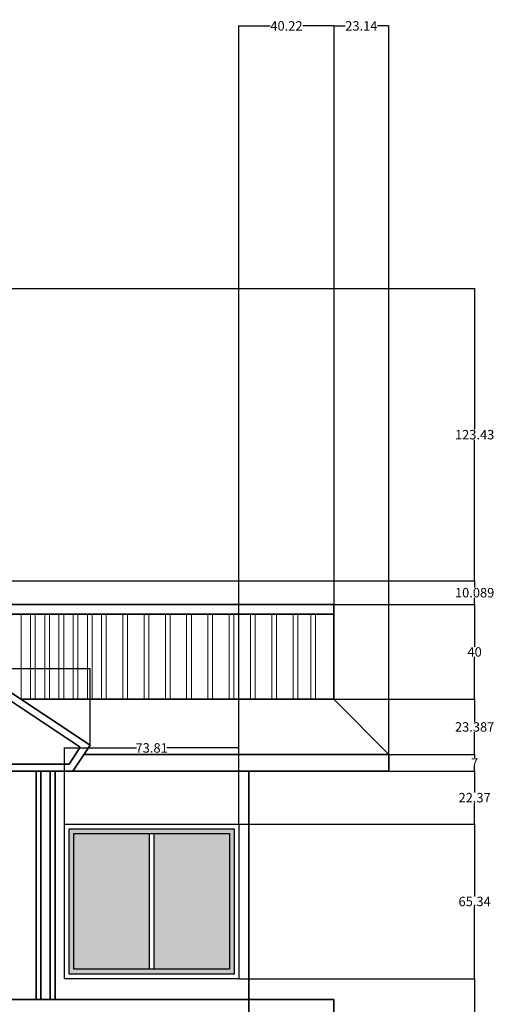
# Model space of a CAD drawing. Units: inches. Extents: x 1366 to 1929, y 372 to 1068.
# Tile 4 of 4: x 1728 to 1929, y 652 to 1068. Entities that reach past the tile are written whole.
import ezdxf

# ---------------------------------------------------------------- set-up
doc = ezdxf.new("R2010")
doc.units = ezdxf.units.IN
doc.header["$MEASUREMENT"] = 0
for name, color, linetype, lineweight in [('A-ANNO-DIMS', 2, 'Continuous', 18), ('A-ELEV', 7, 'Continuous', 35), ('A-ELEV-PATT', 252, 'Continuous', 13), ('A-ELEV-RAIL', 8, 'Continuous', 18), ('A-GLAZ', 4, 'Continuous', 30)]:
    doc.layers.add(name, color=color, linetype=linetype, lineweight=lineweight)
doc.styles.get("Standard").update_dxf_attribs({"font": 'arial.ttf'})
doc.dimstyles.get("Standard").update_dxf_attribs({"dimtxt": 4, "dimasz": 0.18, "dimexe": 0.18, "dimexo": 0.0625, "dimgap": 0.09, "dimtad": 0, "dimtih": 1, "dimtoh": 1, "dimdec": 0, "dimrnd": 6, "dimzin": 0, "dimdsep": 46, "dimlunit": 3, "dimtxsty": 'Standard', "dimcen": 0.09, "dimadec": 0, "dimazin": 0, "dimtfac": 1, "dimtdec": 0, "dimtofl": 0, "dimtmove": 0, "dimatfit": 3, "dimfxl": 1, "dimtolj": 1, "dimtzin": 0, "dimarcsym": 0})

# ---------------------------------------------------------------- blocks, each defined once
blk = doc.blocks.new('*D16')
at = {"layer": 'A-ANNO-DIMS', "color": 0, "lineweight": -2, "transparency": 16777216}
for p, q in [((1820.72, 727.69), (1820.72, 1065.06)), ((1860.94, 820.44), (1860.94, 1065.06)), ((1820.9, 1064.88), (1833.93, 1064.88)), ((1860.76, 1064.88), (1847.73, 1064.88))]:
    blk.add_line(p, q, dxfattribs=at)
at = {"layer": 'A-ANNO-DIMS', "color": 0, "lineweight": 30, "transparency": 16777216}
for points in [[(1820.9, 1064.91), (1820.9, 1064.85), (1820.72, 1064.88)], [(1860.76, 1064.91), (1860.76, 1064.85), (1860.94, 1064.88)]]:
    blk.add_solid(points, dxfattribs=at)
at = {"layer": 'Defpoints', "color": 0, "lineweight": 30, "transparency": 16777216}
for p in [(1860.94, 1064.88), (1860.94, 820.38), (1820.72, 727.62)]:
    blk.add_point(p, dxfattribs=at)
at = {"layer": 'A-ANNO-DIMS', "color": 0, "transparency": 16777216, "insert": (1840.83, 1064.88), "char_height": 4, "attachment_point": 5}
blk.add_mtext('\\A1;40.22', dxfattribs=at)
blk = doc.blocks.new('*D17')
at = {"layer": 'A-ANNO-DIMS', "color": 0, "lineweight": -2, "transparency": 16777216}
for p, q in [((1860.94, 820.44), (1860.94, 1065.06)), ((1884.08, 757.06), (1884.08, 1065.06)), ((1861.12, 1064.88), (1865.64, 1064.88)), ((1883.9, 1064.88), (1879.37, 1064.88))]:
    blk.add_line(p, q, dxfattribs=at)
at = {"layer": 'A-ANNO-DIMS', "color": 0, "lineweight": 30, "transparency": 16777216}
for points in [[(1861.12, 1064.91), (1861.12, 1064.85), (1860.94, 1064.88)], [(1883.9, 1064.91), (1883.9, 1064.85), (1884.08, 1064.88)]]:
    blk.add_solid(points, dxfattribs=at)
at = {"layer": 'Defpoints', "color": 0, "lineweight": 30, "transparency": 16777216}
for p in [(1884.08, 1064.88), (1860.94, 820.38), (1884.08, 756.99)]:
    blk.add_point(p, dxfattribs=at)
at = {"layer": 'A-ANNO-DIMS', "color": 0, "transparency": 16777216, "insert": (1872.51, 1064.88), "char_height": 4, "attachment_point": 5}
blk.add_mtext('\\A1;23.14', dxfattribs=at)
blk = doc.blocks.new('*D43')
at = {"layer": 'A-ANNO-DIMS', "color": 0, "lineweight": -2, "transparency": 16777216}
for p, q in [((1820.78, 662.28), (1920.61, 662.28)), ((1920.43, 662.1), (1920.43, 626.24)), ((1920.43, 586.11), (1920.43, 621.97)), ((1888.28, 585.93), (1920.61, 585.93))]:
    blk.add_line(p, q, dxfattribs=at)
at = {"layer": 'A-ANNO-DIMS', "color": 0, "lineweight": 30, "transparency": 16777216}
for points in [[(1920.4, 662.1), (1920.46, 662.1), (1920.43, 662.28)], [(1920.4, 586.11), (1920.46, 586.11), (1920.43, 585.93)]]:
    blk.add_solid(points, dxfattribs=at)
at = {"layer": 'Defpoints', "color": 0, "lineweight": 30, "transparency": 16777216}
for p in [(1820.72, 662.28), (1920.43, 662.28), (1888.22, 585.93)]:
    blk.add_point(p, dxfattribs=at)
at = {"layer": 'A-ANNO-DIMS', "color": 0, "transparency": 16777216, "insert": (1920.43, 624.11), "char_height": 4, "attachment_point": 5}
blk.add_mtext('\\A1;76.35', dxfattribs=at)
blk = doc.blocks.new('*D44')
at = {"layer": 'A-ANNO-DIMS', "color": 0, "lineweight": -2, "transparency": 16777216}
for p, q in [((1820.78, 727.62), (1920.61, 727.62)), ((1920.43, 727.44), (1920.43, 697.09)), ((1920.43, 662.46), (1920.43, 692.82)), ((1820.78, 662.28), (1920.61, 662.28))]:
    blk.add_line(p, q, dxfattribs=at)
at = {"layer": 'A-ANNO-DIMS', "color": 0, "lineweight": 30, "transparency": 16777216}
for points in [[(1920.4, 727.44), (1920.46, 727.44), (1920.43, 727.62)], [(1920.4, 662.46), (1920.46, 662.46), (1920.43, 662.28)]]:
    blk.add_solid(points, dxfattribs=at)
at = {"layer": 'Defpoints', "color": 0, "lineweight": 30, "transparency": 16777216}
for p in [(1820.72, 727.62), (1920.43, 727.62), (1820.72, 662.28)]:
    blk.add_point(p, dxfattribs=at)
at = {"layer": 'A-ANNO-DIMS', "color": 0, "transparency": 16777216, "insert": (1920.43, 694.95), "char_height": 4, "attachment_point": 5}
blk.add_mtext('\\A1;65.34', dxfattribs=at)
blk = doc.blocks.new('*D45')
at = {"layer": 'A-ANNO-DIMS', "color": 0, "lineweight": -2, "transparency": 16777216}
for p, q in [((1884.14, 749.99), (1920.61, 749.99)), ((1920.43, 749.81), (1920.43, 740.94)), ((1920.43, 727.8), (1920.43, 736.67)), ((1820.78, 727.62), (1920.61, 727.62))]:
    blk.add_line(p, q, dxfattribs=at)
at = {"layer": 'A-ANNO-DIMS', "color": 0, "lineweight": 30, "transparency": 16777216}
for points in [[(1920.4, 749.81), (1920.46, 749.81), (1920.43, 749.99)], [(1920.4, 727.8), (1920.46, 727.8), (1920.43, 727.62)]]:
    blk.add_solid(points, dxfattribs=at)
at = {"layer": 'Defpoints', "color": 0, "lineweight": 30, "transparency": 16777216}
for p in [(1884.08, 749.99), (1920.43, 749.99), (1820.72, 727.62)]:
    blk.add_point(p, dxfattribs=at)
at = {"layer": 'A-ANNO-DIMS', "color": 0, "transparency": 16777216, "insert": (1920.43, 738.81), "char_height": 4, "attachment_point": 5}
blk.add_mtext('\\A1;22.37', dxfattribs=at)
blk = doc.blocks.new('*D46')
at = {"layer": 'A-ANNO-DIMS', "color": 0, "lineweight": -2, "transparency": 16777216}
for p, q in [((1884.139646, 756.992679), (1920.609691, 756.992679)), ((1920.429691, 756.812679), (1920.429691, 755.582679)), ((1884.139646, 749.992679), (1920.609691, 749.992679)), ((1920.429691, 750.172679), (1920.429691, 751.402679))]:
    blk.add_line(p, q, dxfattribs=at)
at = {"layer": 'A-ANNO-DIMS', "color": 0, "lineweight": 30, "transparency": 16777216}
for points in [[(1920.399691, 756.812679), (1920.459691, 756.812679), (1920.429691, 756.992679)], [(1920.399691, 750.172679), (1920.459691, 750.172679), (1920.429691, 749.992679)]]:
    blk.add_solid(points, dxfattribs=at)
at = {"layer": 'Defpoints', "color": 0, "lineweight": 30, "transparency": 16777216}
for p in [(1884.077146, 756.992679), (1920.429691, 756.992679), (1884.077146, 749.992679)]:
    blk.add_point(p, dxfattribs=at)
at = {"layer": 'A-ANNO-DIMS', "color": 0, "transparency": 16777216, "insert": (1920.429691, 753.492679), "char_height": 4, "attachment_point": 5}
blk.add_mtext('\\A1;7', dxfattribs=at)
blk = doc.blocks.new('*D47')
at = {"layer": 'A-ANNO-DIMS', "color": 0, "lineweight": -2, "transparency": 16777216}
for p, q in [((1861, 780.38), (1920.61, 780.38)), ((1920.43, 780.2), (1920.43, 770.82)), ((1920.43, 757.17), (1920.43, 766.55)), ((1884.14, 756.99), (1920.61, 756.99))]:
    blk.add_line(p, q, dxfattribs=at)
at = {"layer": 'A-ANNO-DIMS', "color": 0, "lineweight": 30, "transparency": 16777216}
for points in [[(1920.4, 780.2), (1920.46, 780.2), (1920.43, 780.38)], [(1920.4, 757.17), (1920.46, 757.17), (1920.43, 756.99)]]:
    blk.add_solid(points, dxfattribs=at)
at = {"layer": 'Defpoints', "color": 0, "lineweight": 30, "transparency": 16777216}
for p in [(1860.94, 780.38), (1920.43, 780.38), (1884.08, 756.99)]:
    blk.add_point(p, dxfattribs=at)
at = {"layer": 'A-ANNO-DIMS', "color": 0, "transparency": 16777216, "insert": (1920.43, 768.69), "char_height": 4, "attachment_point": 5}
blk.add_mtext('\\A1;23.387', dxfattribs=at)
blk = doc.blocks.new('*D48')
at = {"layer": 'A-ANNO-DIMS', "color": 0, "lineweight": -2, "transparency": 16777216}
for p, q in [((1861, 820.38), (1920.61, 820.38)), ((1920.43, 820.2), (1920.43, 802.51)), ((1920.43, 780.56), (1920.43, 798.25)), ((1861, 780.38), (1920.61, 780.38))]:
    blk.add_line(p, q, dxfattribs=at)
at = {"layer": 'A-ANNO-DIMS', "color": 0, "lineweight": 30, "transparency": 16777216}
for points in [[(1920.4, 820.2), (1920.46, 820.2), (1920.43, 820.38)], [(1920.4, 780.56), (1920.46, 780.56), (1920.43, 780.38)]]:
    blk.add_solid(points, dxfattribs=at)
at = {"layer": 'Defpoints', "color": 0, "lineweight": 30, "transparency": 16777216}
for p in [(1860.94, 820.38), (1920.43, 820.38), (1860.94, 780.38)]:
    blk.add_point(p, dxfattribs=at)
at = {"layer": 'A-ANNO-DIMS', "color": 0, "transparency": 16777216, "insert": (1920.43, 800.38), "char_height": 4, "attachment_point": 5}
blk.add_mtext('\\A1;40', dxfattribs=at)
blk = doc.blocks.new('*D49')
at = {"layer": 'A-ANNO-DIMS', "color": 0, "lineweight": -2, "transparency": 16777216}
for p, q in [((1652.94, 830.47), (1920.61, 830.47)), ((1920.43, 830.29), (1920.43, 827.56)), ((1861, 820.38), (1920.61, 820.38)), ((1920.43, 820.56), (1920.43, 823.29))]:
    blk.add_line(p, q, dxfattribs=at)
at = {"layer": 'A-ANNO-DIMS', "color": 0, "lineweight": 30, "transparency": 16777216}
for points in [[(1920.4, 830.29), (1920.46, 830.29), (1920.43, 830.47)], [(1920.4, 820.56), (1920.46, 820.56), (1920.43, 820.38)]]:
    blk.add_solid(points, dxfattribs=at)
at = {"layer": 'Defpoints', "color": 0, "lineweight": 30, "transparency": 16777216}
for p in [(1652.88, 830.47), (1920.43, 830.47), (1860.94, 820.38)]:
    blk.add_point(p, dxfattribs=at)
at = {"layer": 'A-ANNO-DIMS', "color": 0, "transparency": 16777216, "insert": (1920.43, 825.42), "char_height": 4, "attachment_point": 5}
blk.add_mtext('\\A1;10.089', dxfattribs=at)
blk = doc.blocks.new('*D50')
at = {"layer": 'A-ANNO-DIMS', "color": 0, "lineweight": -2, "transparency": 16777216}
for p, q in [((1651.18, 953.9), (1920.61, 953.9)), ((1920.43, 953.72), (1920.43, 894.32)), ((1920.43, 830.65), (1920.43, 890.05)), ((1652.94, 830.47), (1920.61, 830.47))]:
    blk.add_line(p, q, dxfattribs=at)
at = {"layer": 'A-ANNO-DIMS', "color": 0, "lineweight": 30, "transparency": 16777216}
for points in [[(1920.4, 953.72), (1920.46, 953.72), (1920.43, 953.9)], [(1920.4, 830.65), (1920.46, 830.65), (1920.43, 830.47)]]:
    blk.add_solid(points, dxfattribs=at)
at = {"layer": 'Defpoints', "color": 0, "lineweight": 30, "transparency": 16777216}
for p in [(1651.11, 953.9), (1920.43, 953.9), (1652.88, 830.47)]:
    blk.add_point(p, dxfattribs=at)
at = {"layer": 'A-ANNO-DIMS', "color": 0, "transparency": 16777216, "insert": (1920.43, 892.18), "char_height": 4, "attachment_point": 5}
blk.add_mtext('\\A1;123.43', dxfattribs=at)
blk = doc.blocks.new('*D51')
at = {"layer": 'A-ANNO-DIMS', "color": 0, "lineweight": -2, "transparency": 16777216}
for p, q in [((1746.91, 727.69), (1746.91, 760)), ((1747.09, 759.82), (1777.38, 759.82)), ((1820.54, 759.82), (1790.25, 759.82)), ((1820.72, 727.69), (1820.72, 760))]:
    blk.add_line(p, q, dxfattribs=at)
at = {"layer": 'A-ANNO-DIMS', "color": 0, "lineweight": 30, "transparency": 16777216}
for points in [[(1747.09, 759.85), (1747.09, 759.79), (1746.91, 759.82)], [(1820.54, 759.85), (1820.54, 759.79), (1820.72, 759.82)]]:
    blk.add_solid(points, dxfattribs=at)
at = {"layer": 'Defpoints', "color": 0, "lineweight": 30, "transparency": 16777216}
for p in [(1820.72, 759.82), (1746.91, 727.62), (1820.72, 727.62)]:
    blk.add_point(p, dxfattribs=at)
at = {"layer": 'A-ANNO-DIMS', "color": 0, "transparency": 16777216, "insert": (1783.81, 759.82), "char_height": 4, "attachment_point": 5}
blk.add_mtext('\\A1;73.81', dxfattribs=at)
blk = doc.blocks.new('*D62')
at = {"layer": 'A-ANNO-DIMS', "color": 0, "lineweight": -2, "transparency": 16777216}
for p, q in [((1547.72, 761.06), (1547.72, 793.37)), ((1547.9, 793.19), (1644.33, 793.19)), ((1757.61, 793.19), (1661.18, 793.19)), ((1757.79, 761.06), (1757.79, 793.37))]:
    blk.add_line(p, q, dxfattribs=at)
at = {"layer": 'A-ANNO-DIMS', "color": 0, "lineweight": 30, "transparency": 16777216}
for points in [[(1547.9, 793.22), (1547.9, 793.16), (1547.72, 793.19)], [(1757.61, 793.22), (1757.61, 793.16), (1757.79, 793.19)]]:
    blk.add_solid(points, dxfattribs=at)
at = {"layer": 'Defpoints', "color": 0, "lineweight": 30, "transparency": 16777216}
for p in [(1757.79, 793.19), (1547.72, 760.99), (1757.79, 760.99)]:
    blk.add_point(p, dxfattribs=at)
at = {"layer": 'A-ANNO-DIMS', "color": 0, "transparency": 16777216, "insert": (1652.75, 793.19), "char_height": 4, "attachment_point": 5}
blk.add_mtext('\\A1;210.06', dxfattribs=at)

msp = doc.modelspace()

# ---------------------------------------------------------------- hatches: boundary and pattern name
at = {"layer": 'A-ELEV-PATT'}
h = msp.add_hatch(color=256, dxfattribs=at)
h.dxf.hatch_style = 1
h.paths.add_polyline_path([(1546.6356, 729.6227), (1468.827, 729.6227), (1468.827, 660.2826), (1546.6356, 660.2826)])
h.paths.add_polyline_path([(1544.6356, 662.2826), (1470.827, 662.2826), (1470.827, 727.6227), (1544.6356, 727.6227)], flags=16)
h.paths.add_polyline_path([(1818.7172, 725.6227), (1748.9085, 725.6227), (1748.9085, 664.2826), (1818.7172, 664.2826)])
h.paths.add_polyline_path([(1750.9085, 723.6227), (1816.7172, 723.6227), (1816.7172, 666.2826), (1750.9085, 666.2826)], flags=16)
h.paths.add_polyline_path([(1546.6356, 895.5665), (1468.827, 895.5665), (1468.827, 826.2264), (1546.6356, 826.2264)])
h.paths.add_polyline_path([(1544.6356, 828.2264), (1470.827, 828.2264), (1470.827, 893.5665), (1544.6356, 893.5665)], flags=16)
h = msp.add_hatch(dxfattribs=at)
h.set_pattern_fill('ANGLE', color=256, scale=25)
h.set_pattern_definition([(0, (0, 0), (0, 6.875), [5, -1.875]), (90, (0, 0), (-6.875, 4e-16), [5, -1.875])])
h.paths.add_polyline_path([(1544.6356, 893.5665), (1508.6356, 893.5665), (1508.6356, 828.2264), (1544.6356, 828.2264)])
h.paths.add_polyline_path([(1506.6356, 727.6227), (1470.827, 727.6227), (1470.827, 662.2826), (1506.6356, 662.2826)])
h.paths.add_polyline_path([(1544.6356, 727.6227), (1508.6356, 727.6227), (1508.6356, 662.2826), (1544.6356, 662.2826)])
h.paths.add_polyline_path([(1608.5338, 752.9927), (1697.2248, 752.9927, 0.93463511)])
h.paths.add_polyline_path([(1682.8585, 567.593), (1622.7881, 567.593), (1622.7881, 535.593), (1682.8585, 535.593)])
h.paths.add_polyline_path([(1782.7172, 723.6227), (1750.9085, 723.6227), (1750.9085, 666.2826), (1782.7172, 666.2826)])
h.paths.add_polyline_path([(1816.7172, 723.6227), (1784.7172, 723.6227), (1784.7172, 666.2826), (1816.7172, 666.2826)])
h.paths.add_polyline_path([(1817.1901, 526.1862), (1739.2847, 526.1862), (1739.2847, 513.1136), (1817.1901, 513.1136)])
h.paths.add_polyline_path([(1565.633, 526.1862), (1487.7276, 526.1862), (1487.7276, 513.1136), (1565.633, 513.1136)])

# ---------------------------------------------------------------- linework, layer by layer
at = {"layer": 'A-ELEV'}
for p, q in [((1652.8793, 830.4686), (1757.7853, 760.9927)), ((1652.8773, 826.8716), (1753.6243, 760.1501)), ((1668.1133, 820.3796), (1860.9351, 820.3796)), ((1860.9351, 820.3796), (1860.9351, 780.3796)), ((1860.9351, 820.3796), (1860.9351, 780.3796)), ((1674.1531, 816.3796), (1860.9351, 816.3796)), ((1728.5118, 780.3796), (1860.9351, 780.3796)), ((1860.9351, 780.3796), (1884.0771, 756.9927)), ((1755.2863, 762.6525), (1755.284, 762.6492)), ((1753.6243, 760.1501), (1748.8704, 752.9927)), ((1757.7853, 760.9927), (1750.4793, 749.9927)), ((1756.1255, 758.4937), (1756.1288, 758.4915)), ((1703.2369, 752.9927), (1748.8704, 752.9927)), ((1755.1285, 756.9927), (1884.0771, 756.9927)), ((1884.0771, 756.9927), (1884.0771, 749.9927)), ((1439.2218, 749.9927), (1860.9351, 749.9927)), ((1734.9351, 749.9927), (1734.9351, 653.5057)), ((1736.9351, 749.9927), (1736.9351, 653.5057)), ((1740.9351, 749.9927), (1740.9351, 653.5057)), ((1742.9351, 749.9927), (1742.9351, 653.5057)), ((1824.9351, 749.9927), (1824.9351, 613.5057)), ((1860.9351, 749.9927), (1884.0771, 749.9927)), ((1439.2218, 653.5057), (1860.9351, 653.5057)), ((1860.9351, 653.5057), (1860.9351, 613.5057))]:
    msp.add_line(p, q, dxfattribs=at)
at = {"layer": 'A-ELEV-RAIL'}
for p, q in [((1728.6001, 816.3796), (1728.6001, 780.3796)), ((1732.6001, 816.3796), (1732.6001, 780.3796)), ((1734.6001, 816.3796), (1734.6001, 780.3796)), ((1738.6001, 816.3796), (1738.6001, 780.3796)), ((1740.6001, 816.3796), (1740.6001, 780.3796)), ((1744.6001, 816.3796), (1744.6001, 780.3796)), ((1746.6001, 816.3796), (1746.6001, 780.3796)), ((1750.6001, 816.3796), (1750.6001, 780.3796)), ((1752.6001, 816.3796), (1752.6001, 780.3796)), ((1756.6001, 816.3796), (1756.6001, 780.3796)), ((1758.6001, 816.3796), (1758.6001, 780.3796)), ((1762.6001, 816.3796), (1762.6001, 780.3796)), ((1764.6001, 816.3796), (1764.6001, 780.3796)), ((1771.6001, 816.3796), (1771.6001, 780.3796)), ((1773.6001, 816.3796), (1773.6001, 780.3796)), ((1780.6001, 816.3796), (1780.6001, 780.3796)), ((1782.6001, 816.3796), (1782.6001, 780.3796)), ((1789.6001, 816.3796), (1789.6001, 780.3796)), ((1791.6001, 816.3796), (1791.6001, 780.3796)), ((1798.6001, 816.3796), (1798.6001, 780.3796)), ((1800.6001, 816.3796), (1800.6001, 780.3796)), ((1807.6001, 816.3796), (1807.6001, 780.3796)), ((1809.6001, 816.3796), (1809.6001, 780.3796)), ((1816.6001, 816.3796), (1816.6001, 780.3796)), ((1818.6001, 816.3796), (1818.6001, 780.3796)), ((1825.6001, 816.3796), (1825.6001, 780.3796)), ((1827.6001, 816.3796), (1827.6001, 780.3796)), ((1834.6001, 816.3796), (1834.6001, 780.3796)), ((1836.6001, 816.3796), (1836.6001, 780.3796)), ((1843.6001, 816.3796), (1843.6001, 780.3796)), ((1845.6001, 816.3796), (1845.6001, 780.3796)), ((1851.1808, 816.3796), (1851.1808, 780.3796)), ((1853.1808, 816.3796), (1853.1808, 780.3796))]:
    msp.add_line(p, q, dxfattribs=at)
at = {"layer": 'A-GLAZ'}
for p, q in [((1782.7172, 723.6227), (1782.7172, 666.2826)), ((1784.7172, 723.6227), (1784.7172, 666.2826))]:
    msp.add_line(p, q, dxfattribs=at)
for points in [[(1820.7172, 727.6227), (1820.7172, 662.2826), (1746.9085, 662.2826), (1746.9085, 727.6227)], [(1818.7172, 725.6227), (1818.7172, 664.2826), (1748.9085, 664.2826), (1748.9085, 725.6227)], [(1816.7172, 723.6227), (1816.7172, 666.2826), (1750.9085, 666.2826), (1750.9085, 723.6227)]]:
    msp.add_lwpolyline(points, close=True, dxfattribs=at)

# ---------------------------------------------------------------- dimensions: what is measured, and where the dimension line sits
at = {"layer": 'A-ANNO-DIMS'}
for base, p1, p2, picture, middle in [((1860.9351, 1064.884), (1820.7172, 727.6227), (1860.9351, 820.3796), '*D16', (1840.8261, 1064.884)), ((1884.0771, 1064.884), (1860.9351, 820.3796), (1884.0771, 756.9927), '*D17', (1872.5061, 1064.884)), ((1757.7853, 793.1927), (1547.7212, 760.9927), (1757.7853, 760.9927), '*D62', (1652.7533, 793.1927)), ((1820.7172, 759.8227), (1746.9085, 727.6227), (1820.7172, 727.6227), '*D51', (1783.8129, 759.8227))]:
    dim = msp.add_linear_dim(base=base, p1=p1, p2=p2, dimstyle='Standard', override={"dimdec": 2, "dimlfac": 1, "dimrnd": 0, "dimzin": 0, "dimdsep": 46, "dimlunit": 2}, dxfattribs=at)
    dim.commit()
    dim.dimension.update_dxf_attribs({"geometry": picture, "text_midpoint": middle})
for base, p1, p2, override, picture, middle in [((1920.4297, 953.8973), (1652.8793, 830.4686), (1651.1133, 953.8973), {"dimdec": 2, "dimlfac": 1, "dimrnd": 0, "dimzin": 0, "dimdsep": 46, "dimlunit": 2}, '*D50', (1920.4297, 892.1829)), ((1920.4297, 830.4686), (1860.9351, 820.3796), (1652.8793, 830.4686), {"dimdec": 3, "dimlfac": 1, "dimrnd": 0, "dimzin": 0, "dimdsep": 46, "dimlunit": 2}, '*D49', (1920.4297, 825.4241)), ((1920.4297, 820.3796), (1860.9351, 780.3796), (1860.9351, 820.3796), {"dimdec": 0, "dimlfac": 1, "dimrnd": 0, "dimzin": 0, "dimdsep": 46, "dimlunit": 2}, '*D48', (1920.4297, 800.3796)), ((1920.4297, 780.3796), (1884.0771, 756.9927), (1860.9351, 780.3796), {"dimdec": 3, "dimlfac": 1, "dimrnd": 0, "dimzin": 0, "dimdsep": 46, "dimlunit": 2}, '*D47', (1920.4297, 768.6861)), ((1920.4297, 756.9927), (1884.0771, 749.9927), (1884.0771, 756.9927), {"dimdec": 0, "dimlfac": 1, "dimrnd": 0, "dimzin": 0, "dimdsep": 46, "dimlunit": 2}, '*D46', (1920.4297, 753.4927)), ((1920.4297, 749.9927), (1820.7172, 727.6227), (1884.0771, 749.9927), {"dimdec": 2, "dimlfac": 1, "dimrnd": 0, "dimzin": 0, "dimdsep": 46, "dimlunit": 2}, '*D45', (1920.4297, 738.8077)), ((1920.4297, 727.6227), (1820.7172, 662.2826), (1820.7172, 727.6227), {"dimdec": 2, "dimlfac": 1, "dimrnd": 0, "dimzin": 0, "dimdsep": 46, "dimlunit": 2}, '*D44', (1920.4297, 694.9526)), ((1920.4297, 662.2826), (1888.2208, 585.9312), (1820.7172, 662.2826), {"dimdec": 2, "dimlfac": 1, "dimrnd": 0, "dimzin": 0, "dimdsep": 46, "dimlunit": 2}, '*D43', (1920.4297, 624.1069))]:
    dim = msp.add_linear_dim(base=base, p1=p1, p2=p2, angle=90, dimstyle='Standard', override=override, dxfattribs=at)
    dim.commit()
    dim.dimension.update_dxf_attribs({"geometry": picture, "text_midpoint": middle})

doc.saveas('drawing.dxf')
